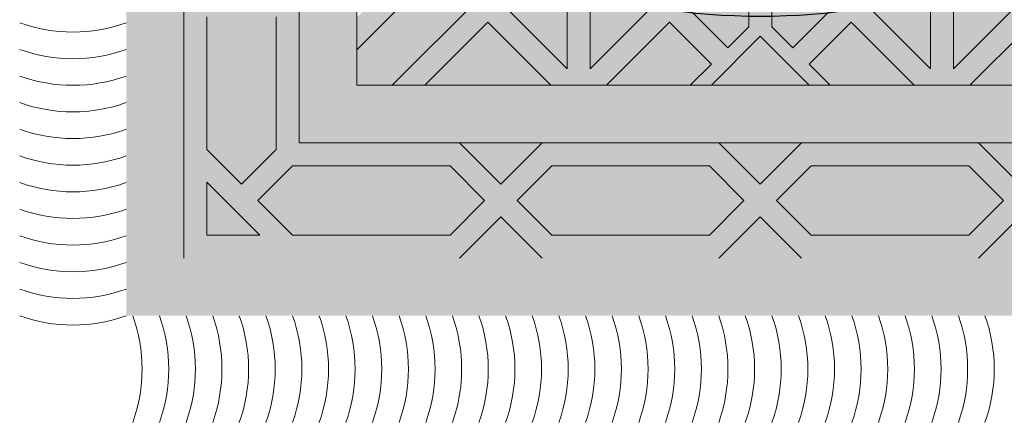
# Model space of a CAD drawing. Units: inches. Extents: x 844 to 2234, y 346 to 1084.
# Tile 26 of 93: x 1249.18 to 1260.07, y 682.93 to 687.38. Entities that reach past the tile are written whole.
import ezdxf

# ---------------------------------------------------------------- set-up
doc = ezdxf.new("R2010")
doc.units = ezdxf.units.IN
doc.header["$MEASUREMENT"] = 0
doc.layers.add('furniture', color=8, linetype='Continuous', lineweight=18)
doc.layers.add('RA-AP-01$0$INT', color=35, linetype='Continuous', lineweight=5)
doc.layers.add('RA-AP-01$0$FURN', color=3, linetype='Continuous')
doc.layers.add('RA-AP-01$0$WOOD', color=64, linetype='Continuous')

# ---------------------------------------------------------------- blocks, each defined once
blk = doc.blocks.new('A$C18D01794')
at = {"layer": 'RA-AP-01$0$INT'}
h = blk.add_hatch(color=256, dxfattribs=at)
h.paths.add_polyline_path([(4.35521, -6.15671), (4.35521, -8.05671), (5.45521, -8.05671), (5.45521, -6.15671)])
h.paths.add_polyline_path([(4.40521, -8.00671), (4.40521, -6.20671), (5.40521, -6.20671), (5.40521, -8.00671)], flags=16)
h = blk.add_hatch(color=256, dxfattribs=at)
h.paths.add_polyline_path([(4.46935, -7.07085), (4.50521, -7.035), (4.50521, -7.10671)])
h.paths.add_polyline_path([(4.45521, -7.085), (4.47692, -7.10671), (4.43349, -7.10671)])
h.paths.add_polyline_path([(4.40521, -7.035), (4.44106, -7.07085), (4.40521, -7.10671)])
h.paths.add_polyline_path([(4.42521, -6.91146), (4.45521, -6.88146), (4.48521, -6.91146), (4.48521, -7.02671), (4.45521, -7.05671), (4.42521, -7.02671)])
h.paths.add_polyline_path([(4.50521, -6.83146), (4.50521, -6.90318), (4.46935, -6.86732)])
h.paths.add_polyline_path([(4.42521, -6.70793), (4.45521, -6.67793), (4.48521, -6.70793), (4.48521, -6.82318), (4.45521, -6.85318), (4.42521, -6.82318)])
h.paths.add_polyline_path([(4.42521, -6.50439), (4.45521, -6.47439), (4.48521, -6.50439), (4.48521, -6.61964), (4.45521, -6.64964), (4.42521, -6.61964)])
h.paths.add_polyline_path([(4.46935, -6.66378), (4.50521, -6.62793), (4.50521, -6.69964)])
h.paths.add_polyline_path([(4.40521, -6.62793), (4.44106, -6.66378), (4.40521, -6.69964)])
h.paths.add_polyline_path([(4.40521, -6.42439), (4.44106, -6.46025), (4.40521, -6.49611)])
h.paths.add_polyline_path([(4.46935, -6.46025), (4.50521, -6.42439), (4.50521, -6.49611)])
h.paths.add_polyline_path([(4.42521, -6.30085), (4.45521, -6.27085), (4.48521, -6.30085), (4.48521, -6.41611), (4.45521, -6.44611), (4.42521, -6.41611)])
h.paths.add_polyline_path([(4.42521, -6.22671), (4.47106, -6.22671), (4.42521, -6.27257)])
h.paths.add_polyline_path([(4.49935, -6.22671), (4.63606, -6.22671), (4.66606, -6.25671), (4.63606, -6.28671), (4.49935, -6.28671), (4.46935, -6.25671)])
h.paths.add_polyline_path([(4.68021, -6.27085), (4.71606, -6.30671), (4.64435, -6.30671)])
h.paths.add_polyline_path([(4.64435, -6.20671), (4.71606, -6.20671), (4.68021, -6.24257)])
h.paths.add_polyline_path([(4.72435, -6.22671), (4.86106, -6.22671), (4.89106, -6.25671), (4.86106, -6.28671), (4.72435, -6.28671), (4.69435, -6.25671)])
h.paths.add_polyline_path([(4.90521, -6.27085), (4.94106, -6.30671), (4.86935, -6.30671)])
h.paths.add_polyline_path([(4.86935, -6.20671), (4.94106, -6.20671), (4.90521, -6.24257)])
h.paths.add_polyline_path([(4.94935, -6.22671), (5.08606, -6.22671), (5.11606, -6.25671), (5.08606, -6.28671), (4.94935, -6.28671), (4.91935, -6.25671)])
h.paths.add_polyline_path([(5.13021, -6.27085), (5.16606, -6.30671), (5.09435, -6.30671)])
h.paths.add_polyline_path([(5.09435, -6.20671), (5.16606, -6.20671), (5.13021, -6.24257)])
h.paths.add_polyline_path([(5.17435, -6.22671), (5.31106, -6.22671), (5.34106, -6.25671), (5.31106, -6.28671), (5.17435, -6.28671), (5.14435, -6.25671)])
h.paths.add_polyline_path([(5.32521, -6.30085), (5.35521, -6.27085), (5.38521, -6.30085), (5.38521, -6.41611), (5.35521, -6.44611), (5.32521, -6.41611)])
h.paths.add_polyline_path([(5.33935, -6.22671), (5.38521, -6.22671), (5.38521, -6.27257)])
h.paths.add_polyline_path([(5.32521, -6.50439), (5.35521, -6.47439), (5.38521, -6.50439), (5.38521, -6.61964), (5.35521, -6.64964), (5.32521, -6.61964)])
h.paths.add_polyline_path([(5.30521, -6.42439), (5.34106, -6.46025), (5.30521, -6.49611)])
h.paths.add_polyline_path([(5.36935, -6.46025), (5.40521, -6.42439), (5.40521, -6.49611)])
h.paths.add_polyline_path([(5.40521, -6.62793), (5.40521, -6.69964), (5.36935, -6.66378)])
h.paths.add_polyline_path([(5.30521, -6.62793), (5.34106, -6.66378), (5.30521, -6.69964)])
h.paths.add_polyline_path([(5.32521, -6.70793), (5.35521, -6.67793), (5.38521, -6.70793), (5.38521, -6.82318), (5.35521, -6.85318), (5.32521, -6.82318)])
h.paths.add_polyline_path([(5.30521, -6.83146), (5.34106, -6.86732), (5.30521, -6.90318)])
h.paths.add_polyline_path([(5.32521, -6.91146), (5.35521, -6.88146), (5.38521, -6.91146), (5.38521, -7.02671), (5.35521, -7.05671), (5.32521, -7.02671)])
h.paths.add_polyline_path([(5.40458, -6.83209, 0.001218), (5.40521, -6.83231), (5.40521, -6.90318), (5.36935, -6.86732)])
h.paths.add_polyline_path([(5.36935, -7.07085), (5.40521, -7.035), (5.40521, -7.10671)])
h.paths.add_polyline_path([(5.35521, -7.085), (5.37692, -7.10671), (5.33349, -7.10671)])
h.paths.add_polyline_path([(5.30521, -7.035), (5.34106, -7.07085), (5.30521, -7.10671)])
h = blk.add_hatch(color=256, dxfattribs=at)
h.paths.add_polyline_path([(4.50521, -6.62793), (4.46935, -6.66378), (4.50521, -6.69964), (4.50521, -6.83146), (4.46935, -6.86732), (4.50521, -6.90318), (4.50521, -7.035), (4.46935, -7.07085), (4.50521, -7.10671), (4.47692, -7.10671), (4.45521, -7.085), (4.43349, -7.10671), (4.40521, -7.10671), (4.44106, -7.07085), (4.40521, -7.035), (4.40521, -6.90318), (4.44106, -6.86732), (4.40521, -6.83146), (4.40521, -6.69964), (4.44106, -6.66378), (4.40521, -6.62793), (4.40521, -6.49611), (4.44106, -6.46025), (4.40521, -6.42439), (4.40521, -6.20671), (4.64435, -6.20671), (4.68021, -6.24257), (4.71606, -6.20671), (4.86935, -6.20671), (4.90521, -6.24257), (4.94106, -6.20671), (5.09435, -6.20671), (5.13021, -6.24257), (5.16606, -6.20671), (5.40521, -6.20671), (5.40521, -6.42439), (5.36935, -6.46025), (5.40521, -6.49611), (5.40521, -6.62793), (5.36935, -6.66378), (5.40521, -6.69964), (5.40521, -6.83146), (5.36935, -6.86732), (5.40521, -6.90318), (5.40521, -7.035), (5.36935, -7.07085), (5.40521, -7.10671), (5.37692, -7.10671), (5.35521, -7.085), (5.33349, -7.10671), (5.30521, -7.10671), (5.34106, -7.07085), (5.30521, -7.035), (5.30521, -6.90318), (5.34106, -6.86732), (5.30521, -6.83146), (5.30521, -6.69964), (5.34106, -6.66378), (5.30521, -6.62793), (5.30521, -6.49611), (5.34106, -6.46025), (5.30521, -6.42439), (5.30521, -6.30671), (5.16606, -6.30671), (5.13021, -6.27085), (5.09435, -6.30671), (4.94106, -6.30671), (4.90521, -6.27085), (4.86935, -6.30671), (4.71606, -6.30671), (4.68021, -6.27085), (4.64435, -6.30671), (4.50521, -6.30671), (4.50521, -6.42439), (4.46935, -6.46025), (4.50521, -6.49611)])
h.paths.add_polyline_path([(4.48521, -6.50439), (4.45521, -6.47439), (4.42521, -6.50439), (4.42521, -6.61964), (4.45521, -6.64964), (4.48521, -6.61964)], flags=16)
h.paths.add_polyline_path([(4.45521, -6.44611), (4.48521, -6.41611), (4.48521, -6.30085), (4.45521, -6.27085), (4.42521, -6.30085), (4.42521, -6.41611)], flags=16)
h.paths.add_polyline_path([(4.45521, -6.67793), (4.42521, -6.70793), (4.42521, -6.82318), (4.45521, -6.85318), (4.48521, -6.82318), (4.48521, -6.70793)], flags=16)
h.paths.add_polyline_path([(4.49935, -6.28671), (4.63606, -6.28671), (4.66606, -6.25671), (4.63606, -6.22671), (4.49935, -6.22671), (4.46935, -6.25671)], flags=16)
h.paths.add_polyline_path([(4.42521, -6.27257), (4.47106, -6.22671), (4.42521, -6.22671)], flags=16)
h.paths.add_polyline_path([(4.45521, -6.88146), (4.42521, -6.91146), (4.42521, -7.02671), (4.45521, -7.05671), (4.48521, -7.02671), (4.48521, -6.91146)], flags=16)
h.paths.add_polyline_path([(4.72435, -6.28671), (4.86106, -6.28671), (4.89106, -6.25671), (4.86106, -6.22671), (4.72435, -6.22671), (4.69435, -6.25671)], flags=16)
h.paths.add_polyline_path([(4.91935, -6.25671), (4.94935, -6.28671), (5.08606, -6.28671), (5.11606, -6.25671), (5.08606, -6.22671), (4.94935, -6.22671)], flags=16)
h.paths.add_polyline_path([(5.14435, -6.25671), (5.17435, -6.28671), (5.31106, -6.28671), (5.34106, -6.25671), (5.31106, -6.22671), (5.17435, -6.22671)], flags=16)
h.paths.add_polyline_path([(5.32521, -6.61964), (5.35521, -6.64964), (5.38521, -6.61964), (5.38521, -6.50439), (5.35521, -6.47439), (5.32521, -6.50439)], flags=16)
h.paths.add_polyline_path([(5.32521, -6.41611), (5.35521, -6.44611), (5.38521, -6.41611), (5.38521, -6.30085), (5.35521, -6.27085), (5.32521, -6.30085)], flags=16)
h.paths.add_polyline_path([(5.32521, -6.70793), (5.32521, -6.82318), (5.35521, -6.85318), (5.38521, -6.82318), (5.38521, -6.70793), (5.35521, -6.67793)], flags=16)
h.paths.add_polyline_path([(5.32521, -6.91146), (5.32521, -7.02671), (5.35521, -7.05671), (5.38521, -7.02671), (5.38521, -6.91146), (5.35521, -6.88146)], flags=16)
h.paths.add_polyline_path([(5.33935, -6.22671), (5.38521, -6.27257), (5.38521, -6.22671)], flags=16)
blk.add_hatch(color=256, dxfattribs=at).paths.add_polyline_path([(4.50521, -6.30671), (5.30521, -6.30671), (5.30521, -7.10671), (5.25521, -7.10671), (5.25521, -6.35671), (4.55521, -6.35671), (4.55521, -7.10671), (4.50521, -7.10671)])
h = blk.add_hatch(color=256, dxfattribs=at)
h.paths.add_polyline_path([(4.58592, -6.35671), (4.55521, -6.35671), (4.55521, -6.38742), (4.8745, -6.70671), (4.90521, -6.676)])
h.paths.add_polyline_path([(5.25521, -6.38742), (5.25521, -6.35671), (5.2245, -6.35671), (4.90521, -6.676), (4.93592, -6.70671)])
h.paths.add_polyline_path([(4.93592, -6.70671), (4.90521, -6.73742), (5.25521, -7.08742), (5.25521, -7.026)])
h.paths.add_polyline_path([(4.55521, -7.026), (4.55521, -7.08742), (4.90521, -6.73742), (4.8745, -6.70671)])
h = blk.add_hatch(color=256, dxfattribs=at)
h.paths.add_polyline_path([(4.58592, -6.35671), (4.6142, -6.35671), (4.66885, -6.41136), (4.72349, -6.35671), (4.77177, -6.35671), (4.82642, -6.41136), (4.86278, -6.375), (4.8445, -6.35671), (4.86278, -6.35671), (4.90521, -6.39914), (4.94763, -6.35671), (4.96592, -6.35671), (4.94763, -6.375), (4.98399, -6.41136), (5.03864, -6.35671), (5.08692, -6.35671), (5.14157, -6.41136), (5.19621, -6.35671), (5.2245, -6.35671), (4.90521, -6.676)])
h.paths.add_polyline_path([(4.89521, -6.63772), (4.89521, -6.52843), (4.84056, -6.58307)], flags=16)
h.paths.add_polyline_path([(4.91521, -6.63772), (4.96985, -6.58307), (4.91521, -6.52843)], flags=16)
h.paths.add_polyline_path([(4.82642, -6.56893), (4.88106, -6.51429), (4.77177, -6.51429)], flags=16)
h.paths.add_polyline_path([(4.98399, -6.56893), (5.03864, -6.51429), (4.92935, -6.51429)], flags=16)
h.paths.add_polyline_path([(4.88106, -6.49429), (4.82642, -6.43964), (4.77177, -6.49429)], flags=16)
h.paths.add_polyline_path([(4.92935, -6.49429), (5.03864, -6.49429), (4.98399, -6.43964)], flags=16)
h.paths.add_polyline_path([(4.89521, -6.48014), (4.89521, -6.40742), (4.87692, -6.38914), (4.84056, -6.4255)], flags=16)
h.paths.add_polyline_path([(4.91521, -6.48014), (4.96985, -6.4255), (4.93349, -6.38914), (4.91521, -6.40742)], flags=16)
h.paths.add_polyline_path([(4.75763, -6.48014), (4.81228, -6.4255), (4.75763, -6.37085)], flags=16)
h.paths.add_polyline_path([(4.73763, -6.48014), (4.73763, -6.37085), (4.68299, -6.4255)], flags=16)
h.paths.add_polyline_path([(5.05278, -6.48014), (5.05278, -6.37085), (4.99814, -6.4255)], flags=16)
h.paths.add_polyline_path([(5.07278, -6.48014), (5.12742, -6.4255), (5.07278, -6.37085)], flags=16)
h.paths.add_polyline_path([(4.93592, -6.70671), (5.25521, -6.38742), (5.25521, -6.41571), (5.20056, -6.47035), (5.25521, -6.525), (5.25521, -6.57328), (5.20056, -6.62793), (5.23692, -6.66429), (5.25521, -6.646), (5.25521, -6.66429), (5.21278, -6.70671), (5.25521, -6.74914), (5.25521, -6.76742), (5.23692, -6.74914), (5.20056, -6.7855), (5.25521, -6.84014), (5.25521, -6.88843), (5.20056, -6.94307), (5.25521, -6.99772), (5.25521, -7.026)])
h.paths.add_polyline_path([(5.04299, -6.7855), (5.09763, -6.84014), (5.09763, -6.73085)], flags=16)
h.paths.add_polyline_path([(5.02885, -6.77136), (5.08349, -6.71671), (4.9742, -6.71671)], flags=16)
h.paths.add_polyline_path([(5.11763, -6.84014), (5.17228, -6.7855), (5.11763, -6.73085)], flags=16)
h.paths.add_polyline_path([(5.08349, -6.69671), (5.02885, -6.64207), (4.9742, -6.69671)], flags=16)
h.paths.add_polyline_path([(5.13177, -6.85429), (5.18642, -6.79964), (5.24106, -6.85429)], flags=17)
h.paths.add_polyline_path([(5.13177, -6.71671), (5.18642, -6.77136), (5.22278, -6.735), (5.2045, -6.71671)], flags=16)
h.paths.add_polyline_path([(5.09763, -6.68257), (5.09763, -6.57328), (5.04299, -6.62793)], flags=16)
h.paths.add_polyline_path([(5.13177, -6.87429), (5.24106, -6.87429), (5.18642, -6.92893)], flags=17)
h.paths.add_polyline_path([(5.13177, -6.69671), (5.2045, -6.69671), (5.22278, -6.67843), (5.18642, -6.64207)], flags=16)
h.paths.add_polyline_path([(5.11763, -6.68257), (5.17228, -6.62793), (5.11763, -6.57328)], flags=16)
h.paths.add_polyline_path([(5.18642, -6.61378), (5.24106, -6.55914), (5.13177, -6.55914)], flags=16)
h.paths.add_polyline_path([(5.13177, -6.53914), (5.24106, -6.53914), (5.18642, -6.48449)], flags=16)
h.paths.add_polyline_path([(5.25521, -7.08742), (5.25521, -7.10671), (4.55521, -7.10671), (4.55521, -7.08742), (4.90521, -6.73742)])
h.paths.add_polyline_path([(4.98399, -6.84449), (4.92935, -6.89914), (5.03864, -6.89914)], flags=16)
h.paths.add_polyline_path([(4.96985, -6.83035), (4.91521, -6.77571), (4.91521, -6.885)], flags=16)
h.paths.add_polyline_path([(4.92935, -6.91914), (4.98399, -6.97378), (5.03864, -6.91914)], flags=16)
h.paths.add_polyline_path([(5.05278, -6.93328), (4.99814, -6.98793), (5.05278, -7.04257)], flags=16)
h.paths.add_polyline_path([(5.07278, -6.93328), (5.07278, -7.04257), (5.12742, -6.98793)], flags=16)
h.paths.add_polyline_path([(4.89521, -6.77571), (4.84056, -6.83035), (4.89521, -6.885)], flags=16)
h.paths.add_polyline_path([(4.91521, -6.93328), (4.91521, -7.006), (4.93349, -7.02429), (4.96985, -6.98793)], flags=16)
h.paths.add_polyline_path([(4.88106, -6.89914), (4.82642, -6.84449), (4.77177, -6.89914)], flags=16)
h.paths.add_polyline_path([(4.89521, -6.93328), (4.84056, -6.98793), (4.87692, -7.02429), (4.89521, -7.006)], flags=16)
h.paths.add_polyline_path([(4.98399, -7.00207), (4.94763, -7.03843), (4.96592, -7.05671), (5.03864, -7.05671)], flags=16)
h.paths.add_polyline_path([(4.88106, -6.91914), (4.77177, -6.91914), (4.82642, -6.97378)], flags=16)
h.paths.add_polyline_path([(4.90521, -7.01429), (4.86278, -7.05671), (4.94763, -7.05671)], flags=16)
h.paths.add_polyline_path([(5.14157, -7.00207), (5.08692, -7.05671), (5.19621, -7.05671)], flags=16)
h.paths.add_polyline_path([(4.82642, -7.00207), (4.77177, -7.05671), (4.8445, -7.05671), (4.86278, -7.03843)], flags=16)
h.paths.add_polyline_path([(4.81228, -6.98793), (4.75763, -6.93328), (4.75763, -7.04257)], flags=16)
h.paths.add_polyline_path([(4.73763, -6.93328), (4.68299, -6.98793), (4.73763, -7.04257)], flags=16)
h.paths.add_polyline_path([(4.72349, -7.05671), (4.66885, -7.00207), (4.6142, -7.05671)], flags=16)
h.paths.add_polyline_path([(4.59763, -6.70671), (4.55521, -6.66429), (4.55521, -6.646), (4.57349, -6.66429), (4.60985, -6.62793), (4.55521, -6.57328), (4.55521, -6.525), (4.60985, -6.47035), (4.55521, -6.41571), (4.55521, -6.38742), (4.8745, -6.70671), (4.55521, -7.026), (4.55521, -6.99772), (4.60985, -6.94307), (4.55521, -6.88843), (4.55521, -6.84014), (4.60985, -6.7855), (4.57349, -6.74914), (4.55521, -6.76742), (4.55521, -6.74914)])
h.paths.add_polyline_path([(4.71278, -6.73085), (4.71278, -6.84014), (4.76742, -6.7855)], flags=16)
h.paths.add_polyline_path([(4.72692, -6.71671), (4.78157, -6.77136), (4.83621, -6.71671)], flags=16)
h.paths.add_polyline_path([(4.69278, -6.73085), (4.63814, -6.7855), (4.69278, -6.84014)], flags=16)
h.paths.add_polyline_path([(4.72692, -6.69671), (4.83621, -6.69671), (4.78157, -6.64207)], flags=16)
h.paths.add_polyline_path([(4.67864, -6.71671), (4.60592, -6.71671), (4.58763, -6.735), (4.62399, -6.77136)], flags=16)
h.paths.add_polyline_path([(4.71278, -6.68257), (4.76742, -6.62793), (4.71278, -6.57328)], flags=16)
h.paths.add_polyline_path([(4.67864, -6.69671), (4.62399, -6.64207), (4.58763, -6.67843), (4.60592, -6.69671)], flags=16)
h.paths.add_polyline_path([(4.69278, -6.68257), (4.69278, -6.57328), (4.63814, -6.62793)], flags=16)
h.paths.add_polyline_path([(4.62399, -6.79964), (4.67864, -6.85429), (4.56935, -6.85429)], flags=17)
h.paths.add_polyline_path([(4.62399, -6.61378), (4.67864, -6.55914), (4.56935, -6.55914)], flags=16)
h.paths.add_polyline_path([(4.67864, -6.87429), (4.62399, -6.92893), (4.56935, -6.87429)], flags=17)
h.paths.add_polyline_path([(4.67864, -6.53914), (4.62399, -6.48449), (4.56935, -6.53914)], flags=16)
h = blk.add_hatch(color=256, dxfattribs=at)
h.paths.add_polyline_path([(4.96985, -6.58307), (4.91521, -6.63772), (4.91521, -6.52843)])
h.paths.add_polyline_path([(4.89521, -6.63772), (4.84056, -6.58307), (4.89521, -6.52843)])
h.paths.add_polyline_path([(4.82642, -6.56893), (4.77177, -6.51429), (4.88106, -6.51429)])
h.paths.add_polyline_path([(4.88106, -6.49429), (4.77177, -6.49429), (4.82642, -6.43964)])
h.paths.add_polyline_path([(4.89521, -6.48014), (4.84056, -6.4255), (4.87692, -6.38914), (4.89521, -6.40742)])
h.paths.add_polyline_path([(4.86278, -6.375), (4.82642, -6.41136), (4.77177, -6.35671), (4.8445, -6.35671)])
h.paths.add_polyline_path([(4.81228, -6.4255), (4.75763, -6.48014), (4.75763, -6.37085)])
h.paths.add_polyline_path([(4.73763, -6.48014), (4.68299, -6.4255), (4.73763, -6.37085)])
h.paths.add_polyline_path([(4.66885, -6.41136), (4.6142, -6.35671), (4.72349, -6.35671)])
h.paths.add_polyline_path([(4.90521, -6.39914), (4.86278, -6.35671), (4.94763, -6.35671)])
h.paths.add_polyline_path([(4.91521, -6.48014), (4.91521, -6.40742), (4.93349, -6.38914), (4.96985, -6.4255)])
h.paths.add_polyline_path([(5.03864, -6.49429), (4.92935, -6.49429), (4.98399, -6.43964)])
h.paths.add_polyline_path([(4.98399, -6.56893), (4.92935, -6.51429), (5.03864, -6.51429)])
h.paths.add_polyline_path([(5.05278, -6.48014), (4.99814, -6.4255), (5.05278, -6.37085)])
h.paths.add_polyline_path([(4.98399, -6.41136), (4.94763, -6.375), (4.96592, -6.35671), (5.03864, -6.35671)])
h.paths.add_polyline_path([(5.12742, -6.4255), (5.07278, -6.48014), (5.07278, -6.37085)])
h.paths.add_polyline_path([(5.14157, -6.41136), (5.08692, -6.35671), (5.19621, -6.35671)])
for p, q in [((4.71606, -6.20671), (4.68021, -6.24257)), ((4.86935, -6.20671), (4.90521, -6.24257)), ((4.94106, -6.20671), (4.90521, -6.24257)), ((5.09435, -6.20671), (5.13021, -6.24257)), ((5.16606, -6.20671), (5.13021, -6.24257)), ((4.72435, -6.22671), (4.69435, -6.25671)), ((4.86106, -6.22671), (4.72435, -6.22671)), ((4.86106, -6.22671), (4.89106, -6.25671)), ((4.94935, -6.22671), (4.91935, -6.25671)), ((4.94935, -6.22671), (5.08606, -6.22671)), ((5.08606, -6.22671), (5.11606, -6.25671)), ((5.17435, -6.22671), (5.14435, -6.25671)), ((5.17435, -6.22671), (5.31106, -6.22671)), ((5.31106, -6.22671), (5.34106, -6.25671)), ((5.33935, -6.22671), (5.38521, -6.27257)), ((5.33935, -6.22671), (5.38521, -6.22671)), ((5.38521, -6.27257), (5.38521, -6.22671)), ((4.72435, -6.28671), (4.69435, -6.25671)), ((4.86106, -6.28671), (4.89106, -6.25671)), ((4.94935, -6.28671), (4.91935, -6.25671)), ((5.08606, -6.28671), (5.11606, -6.25671)), ((5.17435, -6.28671), (5.14435, -6.25671)), ((5.31106, -6.28671), (5.34106, -6.25671)), ((4.71606, -6.30671), (4.68021, -6.27085)), ((4.86935, -6.30671), (4.90521, -6.27085)), ((4.94106, -6.30671), (4.90521, -6.27085)), ((5.09435, -6.30671), (5.13021, -6.27085)), ((5.16606, -6.30671), (5.13021, -6.27085)), ((5.32521, -6.30085), (5.35521, -6.27085)), ((5.38521, -6.30085), (5.35521, -6.27085)), ((4.86106, -6.28671), (4.72435, -6.28671)), ((4.94935, -6.28671), (5.08606, -6.28671)), ((5.17435, -6.28671), (5.31106, -6.28671)), ((5.32521, -6.30085), (5.32521, -6.41611)), ((5.38521, -6.41611), (5.38521, -6.30085)), ((5.26721, -6.30671), (4.54321, -6.30671)), ((5.26721, -6.30671), (4.54321, -6.30671)), ((4.55521, -6.35671), (5.25521, -6.35671)), ((4.72349, -6.35671), (4.66885, -6.41136)), ((4.77177, -6.35671), (4.82642, -6.41136)), ((4.8445, -6.35671), (4.77177, -6.35671)), ((4.8445, -6.35671), (4.86278, -6.375)), ((4.94763, -6.35671), (4.86278, -6.35671)), ((4.90521, -6.39914), (4.86278, -6.35671)), ((4.90521, -6.39914), (4.94763, -6.35671)), ((4.90521, -6.676), (5.2245, -6.35671)), ((4.96592, -6.35671), (4.94763, -6.375)), ((4.94763, -6.375), (4.96592, -6.35671)), ((4.96592, -6.35671), (5.03864, -6.35671)), ((5.03864, -6.35671), (4.98399, -6.41136)), ((5.08692, -6.35671), (5.14157, -6.41136)), ((5.19621, -6.35671), (5.14157, -6.41136)), ((5.25521, -7.10671), (5.25521, -6.35671)), ((4.73763, -6.37085), (4.68299, -6.4255)), ((4.73763, -6.48014), (4.73763, -6.37085)), ((4.75763, -6.48014), (4.75763, -6.37085)), ((4.75763, -6.37085), (4.81228, -6.4255)), ((5.05278, -6.37085), (4.99814, -6.4255)), ((5.05278, -6.48014), (5.05278, -6.37085)), ((5.07278, -6.48014), (5.07278, -6.37085)), ((5.07278, -6.37085), (5.12742, -6.4255)), ((4.82642, -6.41136), (4.86278, -6.375)), ((4.98399, -6.41136), (4.94763, -6.375)), ((4.93592, -6.70671), (5.25521, -6.38742)), ((4.84056, -6.4255), (4.87692, -6.38914)), ((4.89521, -6.40742), (4.87692, -6.38914)), ((4.91521, -6.40742), (4.93349, -6.38914)), ((4.96985, -6.4255), (4.93349, -6.38914)), ((4.89521, -6.40742), (4.89521, -6.48014)), ((4.91521, -6.40742), (4.91521, -6.48014))]:
    blk.add_line(p, q, dxfattribs=at)
for points in [[(5.40521, -7.10671), (5.40521, -6.20671)], [(5.30521, -7.10671), (5.30521, -6.30671), (4.50521, -6.30671), (4.50521, -7.10671)]]:
    blk.add_lwpolyline(points, dxfattribs=at)
for centre, start, end in [((4.83866, -6.11051), 160.20384, 199.79616), ((4.86176, -6.11051), 160.20384, 199.79616), ((4.88486, -6.11051), 160.20384, 199.79616), ((4.90796, -6.11051), 160.20384, 199.79616), ((4.93106, -6.11051), 160.20384, 199.79616), ((4.95416, -6.11051), 160.20384, 199.79616), ((4.97726, -6.11051), 160.20384, 199.79616), ((5.00036, -6.11051), 160.20384, 199.79616), ((5.02346, -6.11051), 160.20384, 199.79616), ((5.04656, -6.11051), 160.20384, 199.79616), ((5.06966, -6.11051), 160.20384, 199.79616), ((5.09276, -6.11051), 160.20384, 199.79616), ((5.11586, -6.11051), 160.20384, 199.79616), ((5.13896, -6.11051), 160.20384, 199.79616), ((5.16206, -6.11051), 160.20384, 199.79616), ((5.18516, -6.11051), 160.20384, 199.79616), ((5.20826, -6.11051), 160.20384, 199.79616), ((5.23136, -6.11051), 160.20384, 199.79616), ((5.25446, -6.11051), 160.20384, 199.79616), ((5.27756, -6.11051), 160.20384, 199.79616), ((5.30066, -6.11051), 160.20384, 199.79616), ((5.32376, -6.11051), 160.20384, 199.79616), ((5.34686, -6.11051), 160.20384, 199.79616), ((5.36996, -6.11051), 160.20384, 199.79616), ((5.39306, -6.11051), 160.20384, 199.79616), ((5.41616, -6.11051), 160.20384, 199.79616), ((5.43926, -6.11051), 160.20384, 199.79616), ((5.46236, -6.11051), 160.20384, 199.79616), ((5.48546, -6.11051), 160.20384, 199.79616), ((5.50856, -6.11051), 160.20384, 199.79616), ((5.53166, -6.11051), 160.20384, 199.79616), ((5.55476, -6.11051), 160.20384, 199.79616), ((5.57786, -6.11051), 160.20384, 199.79616), ((5.50141, -6.28516), 70.20384, 109.79616), ((5.50141, -6.30826), 70.20384, 109.79616), ((5.50141, -6.33136), 70.20384, 109.79616), ((5.50141, -6.35446), 70.20384, 109.79616), ((5.50141, -6.37756), 70.20384, 109.79616), ((5.50141, -6.40066), 70.20384, 109.79616), ((5.50141, -6.42376), 70.20384, 109.79616), ((5.50141, -6.44686), 70.20384, 109.79616), ((5.50141, -6.46996), 70.20384, 109.79616), ((5.50141, -6.49306), 70.20384, 109.79616), ((5.50141, -6.51616), 70.20384, 109.79616), ((5.50141, -6.53926), 70.20384, 109.79616)]:
    blk.add_arc(centre, 0.13641, start, end, dxfattribs=at)
blk = doc.blocks.new('A$C32926AE1')
at = {"layer": 'RA-AP-01$0$WOOD'}
blk.add_arc((4.90477, 4.06706), 0.4604, 252.06839, 287.93161, dxfattribs=at)
blk = doc.blocks.new('A$C5D2F253E')
at = {"layer": 'RA-AP-01$0$FURN', "xscale": -0.7999999999883585, "yscale": 0.7999999999883585, "zscale": 0.8, "rotation": 90}
blk.add_blockref('A$C18D01794', (-5.68776, 4.75792), dxfattribs=at)
at = {"layer": 'RA-AP-01$0$WOOD', "rotation": 270}
blk.add_blockref('A$C32926AE1', (-4.16134, 5.73853), dxfattribs=at)

msp = doc.modelspace()

# ---------------------------------------------------------------- block references
at = {"layer": 'furniture', "xscale": -15.94108302203742, "yscale": 15.94108302203742, "zscale": 15.94108302203742, "rotation": 270}
msp.add_blockref('A$C5D2F253E', (1244.084, 696.258), dxfattribs=at)

doc.saveas('drawing.dxf')
